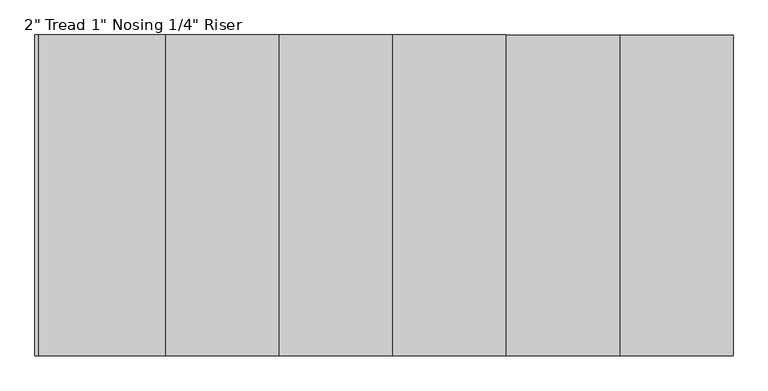
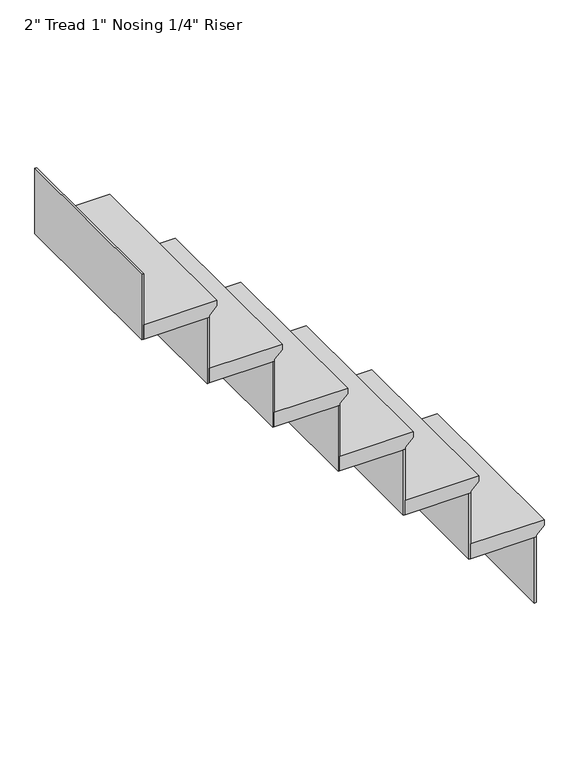
"""IFC4 building model written with IfcOpenShell, lengths in millimetres: stair flight geometry."""

from ifc_helpers import new_model, si_unit, frame, origin, place, context, project, spatial, polyline, outline, extrude, source, transform, mapped, element, save


def stair_flight_f1133b19(model_context):
    return source(origin(), model_context, "Body", "SweptSolid", [
        extrude(outline(polyline([(8229.6, -3295.9634065), (8229.6, -3537.2634065), (8178.8, -3537.2634065), (8178.8, -3321.3634065), (8185.15, -3321.3634065), (8210.55, -3295.9634065), (8229.6, -3295.9634065)])), frame((0.0, 4340.930501, 0.0), z_axis=(0.0, 1.0, 0.0), x_axis=(0.0, 0.0, 1.0)), (0.0, 0.0, 1.0), 609.6),
        extrude(outline(polyline([(-3327.7134065, 4950.530501), (-3321.3634065, 4950.530501), (-3321.3634065, 4340.930501), (-3327.7134065, 4340.930501), (-3327.7134065, 4950.530501)])), frame((0.0, 0.0, 7950.2), z_axis=(0.0, 0.0, 1.0), x_axis=(1.0, 0.0, 0.0)), (0.0, 0.0, 1.0), 228.6),
        extrude(outline(polyline([(-4623.1134065, 4950.530501), (-4616.7634065, 4950.530501), (-4616.7634065, 4340.930501), (-4623.1134065, 4340.930501), (-4623.1134065, 4950.530501)])), frame((0.0, 0.0, 9321.8), z_axis=(0.0, 0.0, 1.0), x_axis=(1.0, 0.0, 0.0)), (0.0, 0.0, 1.0), 228.6),
        extrude(outline(polyline([(-3543.6134065, 4950.530501), (-3537.2634065, 4950.530501), (-3537.2634065, 4340.930501), (-3543.6134065, 4340.930501), (-3543.6134065, 4950.530501)])), frame((0.0, 0.0, 8178.8), z_axis=(0.0, 0.0, 1.0), x_axis=(1.0, 0.0, 0.0)), (0.0, 0.0, 1.0), 228.6),
        extrude(outline(polyline([(8458.2, -3511.8634065), (8458.2, -3753.1634065), (8407.4, -3753.1634065), (8407.4, -3537.2634065), (8413.75, -3537.2634065), (8439.15, -3511.8634065), (8458.2, -3511.8634065)])), frame((0.0, 4340.930501, 0.0), z_axis=(0.0, 1.0, 0.0), x_axis=(0.0, 0.0, 1.0)), (0.0, 0.0, 1.0), 609.6),
        extrude(outline(polyline([(-3759.5134065, 4950.530501), (-3753.1634065, 4950.530501), (-3753.1634065, 4340.930501), (-3759.5134065, 4340.930501), (-3759.5134065, 4950.530501)])), frame((0.0, 0.0, 8407.4), z_axis=(0.0, 0.0, 1.0), x_axis=(1.0, 0.0, 0.0)), (0.0, 0.0, 1.0), 228.6),
        extrude(outline(polyline([(8686.8, -3727.7634065), (8686.8, -3969.0634065), (8636.0, -3969.0634065), (8636.0, -3753.1634065), (8642.35, -3753.1634065), (8667.75, -3727.7634065), (8686.8, -3727.7634065)])), frame((0.0, 4340.930501, 0.0), z_axis=(0.0, 1.0, 0.0), x_axis=(0.0, 0.0, 1.0)), (0.0, 0.0, 1.0), 609.6),
        extrude(outline(polyline([(-3975.4134065, 4950.530501), (-3969.0634065, 4950.530501), (-3969.0634065, 4340.930501), (-3975.4134065, 4340.930501), (-3975.4134065, 4950.530501)])), frame((0.0, 0.0, 8636.0), z_axis=(0.0, 0.0, 1.0), x_axis=(1.0, 0.0, 0.0)), (0.0, 0.0, 1.0), 228.6),
        extrude(outline(polyline([(8915.4, -3943.6634065), (8915.4, -4184.9634065), (8864.6, -4184.9634065), (8864.6, -3969.0634065), (8870.95, -3969.0634065), (8896.35, -3943.6634065), (8915.4, -3943.6634065)])), frame((0.0, 4340.930501, 0.0), z_axis=(0.0, 1.0, 0.0), x_axis=(0.0, 0.0, 1.0)), (0.0, 0.0, 1.0), 609.6),
        extrude(outline(polyline([(-4191.3134065, 4950.530501), (-4184.9634065, 4950.530501), (-4184.9634065, 4340.930501), (-4191.3134065, 4340.930501), (-4191.3134065, 4950.530501)])), frame((0.0, 0.0, 8864.6), z_axis=(0.0, 0.0, 1.0), x_axis=(1.0, 0.0, 0.0)), (0.0, 0.0, 1.0), 228.6),
        extrude(outline(polyline([(9144.0, -4159.5634065), (9144.0, -4400.8634065), (9093.2, -4400.8634065), (9093.2, -4184.9634065), (9099.55, -4184.9634065), (9124.95, -4159.5634065), (9144.0, -4159.5634065)])), frame((0.0, 4340.930501, 0.0), z_axis=(0.0, 1.0, 0.0), x_axis=(0.0, 0.0, 1.0)), (0.0, 0.0, 1.0), 609.6),
        extrude(outline(polyline([(-4407.2134065, 4950.530501), (-4400.8634065, 4950.530501), (-4400.8634065, 4340.930501), (-4407.2134065, 4340.930501), (-4407.2134065, 4950.530501)])), frame((0.0, 0.0, 9093.2), z_axis=(0.0, 0.0, 1.0), x_axis=(1.0, 0.0, 0.0)), (0.0, 0.0, 1.0), 228.6),
        extrude(outline(polyline([(9372.6, -4375.4634065), (9372.6, -4616.7634065), (9321.8, -4616.7634065), (9321.8, -4400.8634065), (9328.15, -4400.8634065), (9353.55, -4375.4634065), (9372.6, -4375.4634065)])), frame((0.0, 4340.930501, 0.0), z_axis=(0.0, 1.0, 0.0), x_axis=(0.0, 0.0, 1.0)), (0.0, 0.0, 1.0), 609.6),
    ])


if __name__ == "__main__":
    model = new_model("IFC4")
    model_context = context("Model", 3, world=origin())
    ifc_project = project(units=[si_unit("LENGTHUNIT", "METRE", prefix="MILLI")], contexts=[model_context])
    site = spatial("IfcSite", under=ifc_project)
    building = spatial("IfcBuilding", under=site)
    placement = place(None, origin())
    stair_flight_shape = stair_flight_f1133b19(model_context)
    element("IfcStairFlight", 1, ObjectType="2\" Tread 1\" Nosing 1/4\" Riser", at=placement, inside=building, context=model_context, shape_type="MappedRepresentation", body=[
        mapped(stair_flight_shape, transform((0.0, 0.0, 0.0), x_axis=(1.0, 0.0, 0.0), y_axis=(0.0, 1.0, 0.0), z_axis=(0.0, 0.0, 1.0))),
    ])
    save(model, "model.ifc")
